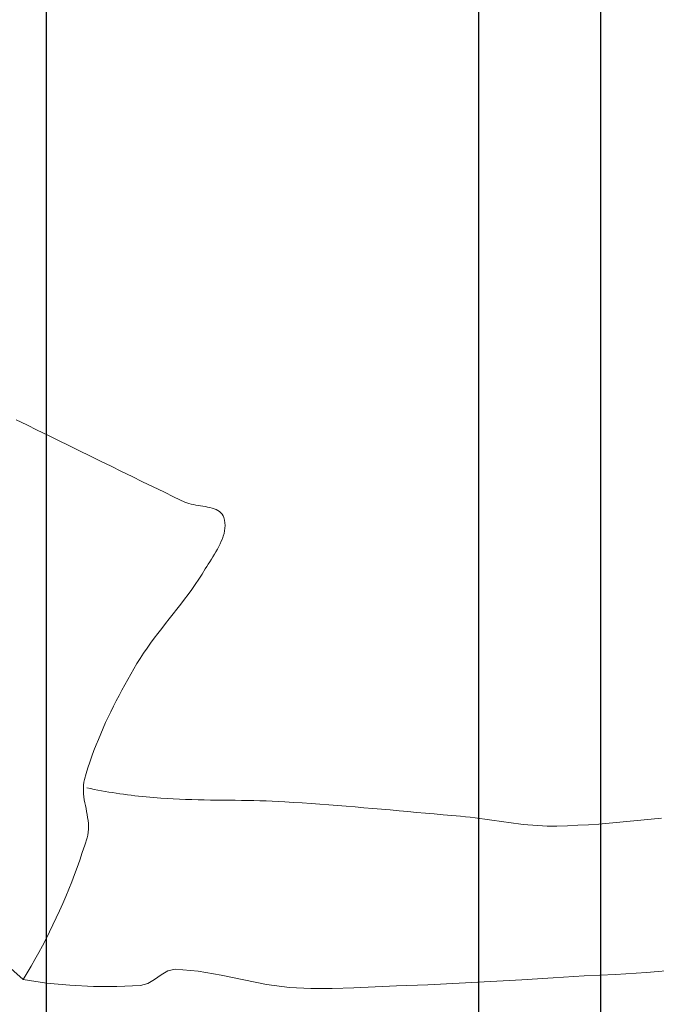
# Model space of a CAD drawing. Units: inches. Extents: x 2656 to 9931, y 1941 to 3068.
# Tile 9 of 46: x 2792 to 2811, y 2502 to 2533. Entities that reach past the tile are written whole.
import ezdxf

# ---------------------------------------------------------------- set-up
doc = ezdxf.new("R2010")
doc.units = ezdxf.units.IN
doc.layers.add('A-ANNO-DIMS', color=2, linetype='Continuous', lineweight=18)
doc.layers.add('A-FURN', color=8, linetype='Continuous', lineweight=13)
doc.styles.get("Standard").update_dxf_attribs({"font": 'arial.ttf'})
doc.dimstyles.new('ISO-25', dxfattribs={"dimtxt": 6, "dimasz": 2.5, "dimexe": 1.25, "dimexo": 0.625, "dimtad": 1, "dimdec": 0, "dimlunit": 3, "dimtxsty": 'Standard', "dimcen": 2.5, "dimadec": 0, "dimazin": 0, "dimtfac": 1, "dimtdec": 0, "dimtmove": 0, "dimatfit": 3, "dimfxl": 1, "dimarcsym": 0})

# ---------------------------------------------------------------- blocks, each defined once
blk = doc.blocks.new('BED-DOUBLE')
for p, q in [((38.504, 17.505), (38.175, 17.662)), ((38.832, 17.346), (38.504, 17.505)), ((39.16, 17.186), (38.832, 17.346)), ((39.488, 17.026), (39.16, 17.186)), ((39.816, 16.865), (39.488, 17.026)), ((40.143, 16.704), (39.816, 16.865)), ((40.47, 16.542), (40.143, 16.704)), ((40.797, 16.381), (40.47, 16.542)), ((41.125, 16.22), (40.797, 16.381)), ((41.452, 16.059), (41.125, 16.22)), ((41.78, 15.898), (41.452, 16.059)), ((42.107, 15.738), (41.78, 15.898)), ((42.436, 15.579), (42.107, 15.738)), ((42.764, 15.421), (42.436, 15.579)), ((43.094, 15.263), (42.764, 15.421)), ((43.424, 15.108), (43.094, 15.263)), ((43.485, 15.082), (43.424, 15.108)), ((43.55, 15.06), (43.485, 15.082)), ((43.618, 15.042), (43.55, 15.06)), ((43.689, 15.026), (43.618, 15.042)), ((43.762, 15.012), (43.689, 15.026)), ((43.836, 15), (43.762, 15.012)), ((43.91, 14.988), (43.836, 15)), ((43.985, 14.977), (43.91, 14.988)), ((44.059, 14.965), (43.985, 14.977)), ((44.131, 14.952), (44.059, 14.965)), ((44.201, 14.937), (44.131, 14.952)), ((44.269, 14.92), (44.201, 14.937)), ((44.333, 14.899), (44.269, 14.92)), ((44.394, 14.876), (44.333, 14.899)), ((44.45, 14.848), (44.394, 14.876)), ((44.501, 14.815), (44.45, 14.848)), ((44.545, 14.776), (44.501, 14.815)), ((44.584, 14.732), (44.545, 14.776)), ((44.615, 14.68), (44.584, 14.732)), ((44.638, 14.622), (44.615, 14.68)), ((44.658, 14.541), (44.638, 14.622)), ((44.67, 14.459), (44.658, 14.541)), ((44.673, 14.377), (44.67, 14.459)), ((44.617, 14.049), (44.64, 14.131)), ((44.64, 14.131), (44.658, 14.213)), ((44.658, 14.213), (44.669, 14.295)), ((44.669, 14.295), (44.673, 14.377)), ((44.478, 13.723), (44.519, 13.804)), ((44.519, 13.804), (44.556, 13.885)), ((44.556, 13.885), (44.588, 13.967)), ((44.588, 13.967), (44.617, 14.049)), ((44.294, 13.405), (44.342, 13.484)), ((44.342, 13.484), (44.389, 13.563)), ((44.389, 13.563), (44.435, 13.643)), ((44.435, 13.643), (44.478, 13.723)), ((44.103, 13.101), (44.149, 13.175)), ((44.149, 13.175), (44.197, 13.251)), ((44.197, 13.251), (44.246, 13.328)), ((44.246, 13.328), (44.294, 13.405)), ((43.958, 12.864), (44.058, 13.027)), ((44.058, 13.027), (44.103, 13.101)), ((43.747, 12.546), (43.854, 12.704)), ((43.854, 12.704), (43.958, 12.864)), ((43.524, 12.235), (43.637, 12.389)), ((43.637, 12.389), (43.747, 12.546)), ((43.293, 11.929), (43.409, 12.081)), ((43.409, 12.081), (43.524, 12.235)), ((43.057, 11.626), (43.175, 11.777)), ((43.175, 11.777), (43.293, 11.929)), ((42.82, 11.325), (42.938, 11.476)), ((42.938, 11.476), (43.057, 11.626)), ((42.585, 11.021), (42.702, 11.173)), ((42.702, 11.173), (42.82, 11.325)), ((42.356, 10.714), (42.469, 10.869)), ((42.469, 10.869), (42.585, 11.021)), ((42.136, 10.401), (42.245, 10.559)), ((42.245, 10.559), (42.356, 10.714)), ((41.93, 10.08), (42.031, 10.242)), ((42.031, 10.242), (42.136, 10.401)), ((41.739, 9.752), (41.832, 9.915)), ((41.832, 9.915), (41.93, 10.08)), ((41.555, 9.422), (41.647, 9.587)), ((41.647, 9.587), (41.739, 9.752)), ((41.377, 9.089), (41.465, 9.256)), ((41.465, 9.256), (41.555, 9.422)), ((41.204, 8.753), (41.289, 8.921)), ((41.289, 8.921), (41.377, 9.089)), ((41.038, 8.413), (41.12, 8.583)), ((41.12, 8.583), (41.204, 8.753)), ((40.958, 8.242), (41.038, 8.413)), ((40.805, 7.896), (40.88, 8.069)), ((40.88, 8.069), (40.958, 8.242)), ((40.661, 7.547), (40.732, 7.722)), ((40.732, 7.722), (40.805, 7.896)), ((40.529, 7.195), (40.594, 7.371)), ((40.594, 7.371), (40.661, 7.547)), ((40.467, 7.017), (40.529, 7.195)), ((40.353, 6.658), (40.408, 6.838)), ((40.408, 6.838), (40.467, 7.017)), ((40.281, 6.389), (40.301, 6.477)), ((40.301, 6.477), (40.353, 6.658)), ((40.264, 6.21), (40.269, 6.3)), ((40.264, 6.119), (40.264, 6.21)), ((40.269, 6.3), (40.281, 6.389)), ((40.368, 6.212), (40.482, 6.189)), ((40.482, 6.189), (40.596, 6.166)), ((40.596, 6.166), (40.711, 6.144)), ((40.711, 6.144), (40.826, 6.123)), ((40.27, 6.028), (40.264, 6.119)), ((40.281, 5.936), (40.27, 6.028)), ((40.294, 5.844), (40.281, 5.936)), ((40.31, 5.751), (40.294, 5.844)), ((40.826, 6.123), (40.941, 6.103)), ((40.941, 6.103), (41.056, 6.083)), ((41.056, 6.083), (41.171, 6.064)), ((41.171, 6.064), (41.286, 6.046)), ((41.286, 6.046), (41.402, 6.029)), ((41.402, 6.029), (41.517, 6.012)), ((41.517, 6.012), (41.633, 5.997)), ((41.633, 5.997), (41.749, 5.982)), ((41.749, 5.982), (41.864, 5.968)), ((41.864, 5.968), (41.98, 5.954)), ((41.98, 5.954), (42.096, 5.942)), ((42.096, 5.942), (42.213, 5.93)), ((42.213, 5.93), (42.329, 5.919)), ((42.329, 5.919), (42.445, 5.909)), ((42.445, 5.909), (42.561, 5.899)), ((42.561, 5.899), (42.677, 5.891)), ((42.677, 5.891), (42.87, 5.878)), ((42.87, 5.878), (43.062, 5.868)), ((43.062, 5.868), (43.254, 5.859)), ((43.254, 5.859), (43.447, 5.852)), ((43.447, 5.852), (43.639, 5.846)), ((43.639, 5.846), (43.832, 5.841)), ((43.832, 5.841), (44.024, 5.838)), ((44.024, 5.838), (44.217, 5.834)), ((44.217, 5.834), (44.41, 5.832)), ((44.41, 5.832), (44.602, 5.83)), ((44.602, 5.83), (44.795, 5.828)), ((44.795, 5.828), (44.988, 5.825)), ((44.988, 5.825), (45.18, 5.823)), ((45.18, 5.823), (45.373, 5.82)), ((40.328, 5.659), (40.31, 5.751)), ((40.347, 5.566), (40.328, 5.659)), ((40.365, 5.473), (40.347, 5.566)), ((45.373, 5.82), (45.566, 5.816)), ((45.566, 5.816), (45.758, 5.811)), ((45.758, 5.811), (45.951, 5.805)), ((45.951, 5.805), (46.143, 5.798)), ((46.143, 5.798), (46.336, 5.789)), ((46.336, 5.789), (46.528, 5.778)), ((46.528, 5.778), (46.802, 5.761)), ((46.802, 5.761), (47.076, 5.743)), ((47.076, 5.743), (47.35, 5.724)), ((47.35, 5.724), (47.624, 5.705)), ((47.624, 5.705), (47.898, 5.684)), ((47.898, 5.684), (48.172, 5.663)), ((48.172, 5.663), (48.445, 5.641)), ((48.445, 5.641), (48.719, 5.619)), ((48.719, 5.619), (48.993, 5.596)), ((48.993, 5.596), (49.266, 5.573)), ((49.266, 5.573), (49.54, 5.549)), ((49.54, 5.549), (49.813, 5.525)), ((49.813, 5.525), (50.087, 5.5)), ((40.382, 5.381), (40.365, 5.473)), ((40.398, 5.288), (40.382, 5.381)), ((40.411, 5.196), (40.398, 5.288)), ((50.087, 5.5), (50.36, 5.476)), ((50.36, 5.476), (50.634, 5.451)), ((50.634, 5.451), (50.907, 5.426)), ((50.907, 5.426), (51.181, 5.402)), ((51.181, 5.402), (51.454, 5.377)), ((51.454, 5.377), (51.728, 5.352)), ((51.728, 5.352), (52.002, 5.328)), ((52.002, 5.328), (52.151, 5.313)), ((52.151, 5.313), (52.301, 5.297)), ((52.301, 5.297), (52.451, 5.279)), ((52.451, 5.279), (52.601, 5.26)), ((52.601, 5.26), (52.75, 5.239)), ((52.75, 5.239), (52.9, 5.218)), ((52.9, 5.218), (53.05, 5.197)), ((57.605, 5.207), (57.93, 5.241)), ((57.93, 5.241), (58.256, 5.275)), ((40.42, 5.105), (40.411, 5.196)), ((40.416, 4.834), (40.424, 4.924)), ((40.424, 5.014), (40.42, 5.105)), ((40.424, 4.924), (40.424, 5.014)), ((53.05, 5.197), (53.199, 5.176)), ((53.199, 5.176), (53.349, 5.155)), ((53.349, 5.155), (53.498, 5.134)), ((53.498, 5.134), (53.648, 5.114)), ((53.648, 5.114), (53.798, 5.095)), ((53.798, 5.095), (53.947, 5.078)), ((53.947, 5.078), (54.097, 5.062)), ((54.097, 5.062), (54.247, 5.049)), ((54.247, 5.049), (54.397, 5.038)), ((54.397, 5.038), (54.547, 5.029)), ((54.547, 5.029), (54.697, 5.024)), ((54.697, 5.024), (54.847, 5.021)), ((54.847, 5.021), (54.998, 5.023)), ((54.998, 5.023), (55.324, 5.032)), ((55.324, 5.032), (55.651, 5.047)), ((55.651, 5.047), (55.977, 5.065)), ((55.977, 5.065), (56.303, 5.088)), ((56.303, 5.088), (56.628, 5.114)), ((56.628, 5.114), (56.954, 5.143)), ((56.954, 5.143), (57.279, 5.174)), ((57.279, 5.174), (57.605, 5.207)), ((40.307, 4.427), (40.38, 4.658)), ((40.38, 4.658), (40.402, 4.746)), ((40.402, 4.746), (40.416, 4.834)), ((40.232, 4.197), (40.307, 4.427)), ((40.154, 3.968), (40.232, 4.197)), ((39.988, 3.512), (40.072, 3.739)), ((40.072, 3.739), (40.154, 3.968)), ((39.901, 3.285), (39.988, 3.512)), ((39.811, 3.06), (39.901, 3.285)), ((39.623, 2.612), (39.718, 2.835)), ((39.718, 2.835), (39.811, 3.06)), ((39.524, 2.39), (39.623, 2.612)), ((39.319, 1.949), (39.423, 2.169)), ((39.423, 2.169), (39.524, 2.39)), ((39.213, 1.731), (39.319, 1.949)), ((39.103, 1.515), (39.213, 1.731)), ((38.876, 1.085), (38.991, 1.299)), ((38.991, 1.299), (39.103, 1.515)), ((37.459, 1.078), (38.392, 0.247)), ((38.759, 0.873), (38.876, 1.085)), ((38.517, 0.454), (38.639, 0.663)), ((38.639, 0.663), (38.759, 0.873)), ((38.392, 0.247), (38.517, 0.454)), ((42.478, 0.252), (42.684, 0.399)), ((42.684, 0.399), (42.897, 0.52)), ((42.897, 0.52), (43.125, 0.568)), ((43.125, 0.568), (43.84, 0.512)), ((43.84, 0.512), (44.549, 0.388)), ((44.549, 0.388), (45.256, 0.236)), ((54.881, 0.304), (55.85, 0.359)), ((55.85, 0.359), (56.819, 0.409)), ((56.819, 0.409), (57.788, 0.467)), ((57.788, 0.467), (58.754, 0.547)), ((38.392, 0.247), (39.115, 0.14)), ((39.115, 0.14), (39.844, 0.068)), ((39.844, 0.068), (40.575, 0.031)), ((40.575, 0.031), (41.307, 0.028)), ((41.307, 0.028), (42.038, 0.06)), ((42.038, 0.06), (42.266, 0.124)), ((42.266, 0.124), (42.478, 0.252)), ((45.256, 0.236), (45.964, 0.094)), ((45.964, 0.094), (46.677, 0.002)), ((46.677, 0.002), (47.342, -0.03)), ((48.675, -0.01), (49.342, 0.02)), ((49.342, 0.02), (50.009, 0.048)), ((50.009, 0.048), (50.984, 0.088)), ((50.984, 0.088), (51.958, 0.135)), ((51.958, 0.135), (52.933, 0.187)), ((52.933, 0.187), (53.907, 0.244)), ((53.907, 0.244), (54.881, 0.304)), ((47.342, -0.03), (48.009, -0.03)), ((48.009, -0.03), (48.675, -0.01))]:
    blk.add_line(p, q)
blk = doc.blocks.new('*D31')
at = {"layer": 'A-ANNO-DIMS', "color": 0, "lineweight": -2, "transparency": 16777216}
for p, q in [((2753.358, 2502.145), (2753.358, 2488.227)), ((2841.982, 2502.145), (2841.982, 2488.227)), ((2755.858, 2489.477), (2839.482, 2489.477)), ((2841.982, 2489.477), (2952.348, 2489.477))]:
    blk.add_line(p, q, dxfattribs=at)
at = {"layer": 'A-ANNO-DIMS', "color": 0, "transparency": 16777216}
for points in [[(2755.858, 2489.893), (2755.858, 2489.06), (2753.358, 2489.477)], [(2839.482, 2489.893), (2839.482, 2489.06), (2841.982, 2489.477)]]:
    blk.add_solid(points, dxfattribs=at)
at = {"layer": 'Defpoints', "color": 0, "transparency": 16777216}
for p in [(2753.358, 2502.77), (2841.982, 2502.77), (2841.982, 2489.477)]:
    blk.add_point(p, dxfattribs=at)
at = {"layer": 'A-ANNO-DIMS', "color": 0, "transparency": 16777216, "insert": (2898.415, 2493.206), "char_height": 6, "attachment_point": 5}
blk.add_mtext('DOUBLE BED 7\'-4 1/2" TYP.', dxfattribs=at)
blk = doc.blocks.new('*D113')
at = {"layer": 'A-ANNO-DIMS', "color": 0, "lineweight": -2, "transparency": 16777216}
for p, q in [((2752.157, 2300.725), (2752.157, 2674.45)), ((2809.769, 2300.725), (2809.769, 2674.45)), ((2754.657, 2673.2), (2807.269, 2673.2))]:
    blk.add_line(p, q, dxfattribs=at)
at = {"layer": 'A-ANNO-DIMS', "color": 0, "transparency": 16777216}
for points in [[(2754.657, 2673.617), (2754.657, 2672.784), (2752.157, 2673.2)], [(2807.269, 2673.617), (2807.269, 2672.784), (2809.769, 2673.2)]]:
    blk.add_solid(points, dxfattribs=at)
at = {"layer": 'Defpoints', "color": 0, "transparency": 16777216}
for p in [(2809.769, 2673.2), (2752.157, 2300.1), (2809.769, 2300.1)]:
    blk.add_point(p, dxfattribs=at)
at = {"layer": 'A-ANNO-DIMS', "color": 0, "transparency": 16777216, "insert": (2780.963, 2676.928), "char_height": 6, "attachment_point": 5}
blk.add_mtext('4\'-9 1/2"', dxfattribs=at)
blk = doc.blocks.new('*D114')
at = {"layer": 'A-ANNO-DIMS', "color": 0, "lineweight": -2, "transparency": 16777216}
for p, q in [((2809.769, 2300.725), (2809.769, 2674.45)), ((2851.877, 2300.725), (2851.877, 2674.45)), ((2812.269, 2673.2), (2849.377, 2673.2))]:
    blk.add_line(p, q, dxfattribs=at)
at = {"layer": 'A-ANNO-DIMS', "color": 0, "transparency": 16777216}
for points in [[(2812.269, 2673.617), (2812.269, 2672.784), (2809.769, 2673.2)], [(2849.377, 2673.617), (2849.377, 2672.784), (2851.877, 2673.2)]]:
    blk.add_solid(points, dxfattribs=at)
at = {"layer": 'Defpoints', "color": 0, "transparency": 16777216}
for p in [(2851.877, 2673.2), (2809.769, 2300.1), (2851.877, 2300.1)]:
    blk.add_point(p, dxfattribs=at)
at = {"layer": 'A-ANNO-DIMS', "color": 0, "transparency": 16777216, "insert": (2830.823, 2676.891), "char_height": 6, "attachment_point": 5}
blk.add_mtext('3\'-6"', dxfattribs=at)
blk = doc.blocks.new('*D129')
at = {"layer": 'A-ANNO-DIMS', "color": 0, "lineweight": -2, "transparency": 16777216}
for p, q in [((2752.157, 2601.146), (2752.157, 2009.273)), ((2777.587, 2557.74), (2777.587, 2009.273)), ((2754.657, 2010.523), (2775.087, 2010.523)), ((2777.587, 2010.523), (2811.37, 2010.523))]:
    blk.add_line(p, q, dxfattribs=at)
at = {"layer": 'A-ANNO-DIMS', "color": 0, "transparency": 16777216}
for points in [[(2754.657, 2010.939), (2754.657, 2010.106), (2752.157, 2010.523)], [(2775.087, 2010.939), (2775.087, 2010.106), (2777.587, 2010.523)]]:
    blk.add_solid(points, dxfattribs=at)
at = {"layer": 'Defpoints', "color": 0, "transparency": 16777216}
for p in [(2752.157, 2601.771), (2777.587, 2558.365), (2777.587, 2010.523)]:
    blk.add_point(p, dxfattribs=at)
at = {"layer": 'A-ANNO-DIMS', "color": 0, "transparency": 16777216, "insert": (2795.728, 2014.25), "char_height": 6, "attachment_point": 5}
blk.add_mtext('2\'-1 1/2"', dxfattribs=at)
blk = doc.blocks.new('*D132')
at = {"layer": 'A-ANNO-DIMS', "color": 0, "lineweight": -2, "transparency": 16777216}
for p, q in [((2763.467, 2366.557), (2763.467, 2674.45)), ((2805.965, 2366.557), (2805.965, 2674.45)), ((2765.967, 2673.2), (2803.465, 2673.2))]:
    blk.add_line(p, q, dxfattribs=at)
at = {"layer": 'A-ANNO-DIMS', "color": 0, "transparency": 16777216}
for points in [[(2765.967, 2673.617), (2765.967, 2672.784), (2763.467, 2673.2)], [(2803.465, 2673.617), (2803.465, 2672.784), (2805.965, 2673.2)]]:
    blk.add_solid(points, dxfattribs=at)
at = {"layer": 'Defpoints', "color": 0, "transparency": 16777216}
for p in [(2805.965, 2673.2), (2763.467, 2365.932), (2805.965, 2365.932)]:
    blk.add_point(p, dxfattribs=at)
at = {"layer": 'A-ANNO-DIMS', "color": 0, "transparency": 16777216, "insert": (2784.716, 2676.93), "char_height": 6, "attachment_point": 5}
blk.add_mtext('3\'-6 1/2"', dxfattribs=at)
blk = doc.blocks.new('*D134')
at = {"layer": 'A-ANNO-DIMS', "color": 0, "lineweight": -2, "transparency": 16777216}
for p, q in [((2752.157, 2300.725), (2752.157, 2674.45)), ((2763.467, 2347.433), (2763.467, 2674.45)), ((2754.657, 2673.2), (2760.967, 2673.2)), ((2763.467, 2673.2), (2801.809, 2673.2))]:
    blk.add_line(p, q, dxfattribs=at)
at = {"layer": 'A-ANNO-DIMS', "color": 0, "transparency": 16777216}
for points in [[(2754.657, 2673.617), (2754.657, 2672.784), (2752.157, 2673.2)], [(2760.967, 2673.617), (2760.967, 2672.784), (2763.467, 2673.2)]]:
    blk.add_solid(points, dxfattribs=at)
at = {"layer": 'Defpoints', "color": 0, "transparency": 16777216}
for p in [(2763.467, 2673.2), (2763.467, 2346.808), (2752.157, 2300.1)]:
    blk.add_point(p, dxfattribs=at)
at = {"layer": 'A-ANNO-DIMS', "color": 0, "transparency": 16777216, "insert": (2783.888, 2676.928), "char_height": 6, "attachment_point": 5}
blk.add_mtext('0\'-11 1/2"', dxfattribs=at)
blk = doc.blocks.new('*D136')
at = {"layer": 'A-ANNO-DIMS', "color": 0, "lineweight": -2, "transparency": 16777216}
for p, q in [((2765.357, 2375.042), (2765.357, 2674.45)), ((2779.142, 2375.042), (2779.142, 2674.45)), ((2767.857, 2673.2), (2776.642, 2673.2)), ((2779.142, 2673.2), (2798.277, 2673.2))]:
    blk.add_line(p, q, dxfattribs=at)
at = {"layer": 'A-ANNO-DIMS', "color": 0, "transparency": 16777216}
for points in [[(2767.857, 2673.617), (2767.857, 2672.784), (2765.357, 2673.2)], [(2776.642, 2673.617), (2776.642, 2672.784), (2779.142, 2673.2)]]:
    blk.add_solid(points, dxfattribs=at)
at = {"layer": 'Defpoints', "color": 0, "transparency": 16777216}
for p in [(2779.142, 2673.2), (2765.357, 2374.417), (2779.142, 2374.417)]:
    blk.add_point(p, dxfattribs=at)
at = {"layer": 'A-ANNO-DIMS', "color": 0, "transparency": 16777216, "insert": (2789.959, 2676.838), "char_height": 6, "attachment_point": 5}
blk.add_mtext('1\'-2"', dxfattribs=at)
blk = doc.blocks.new('*D137')
at = {"layer": 'A-ANNO-DIMS', "color": 0, "lineweight": -2, "transparency": 16777216}
for p, q in [((2779.142, 2375.042), (2779.142, 2674.45)), ((2792.516, 2375.042), (2792.516, 2674.45)), ((2781.642, 2673.2), (2790.016, 2673.2)), ((2792.516, 2673.2), (2825.632, 2673.2))]:
    blk.add_line(p, q, dxfattribs=at)
at = {"layer": 'A-ANNO-DIMS', "color": 0, "transparency": 16777216}
for points in [[(2781.642, 2673.617), (2781.642, 2672.784), (2779.142, 2673.2)], [(2790.016, 2673.617), (2790.016, 2672.784), (2792.516, 2673.2)]]:
    blk.add_solid(points, dxfattribs=at)
at = {"layer": 'Defpoints', "color": 0, "transparency": 16777216}
for p in [(2792.516, 2673.2), (2779.142, 2374.417), (2792.516, 2374.417)]:
    blk.add_point(p, dxfattribs=at)
at = {"layer": 'A-ANNO-DIMS', "color": 0, "transparency": 16777216, "insert": (2810.324, 2676.928), "char_height": 6, "attachment_point": 5}
blk.add_mtext('1\'-1 1/2"', dxfattribs=at)

msp = doc.modelspace()

# ---------------------------------------------------------------- block references
at = {"layer": 'A-FURN'}
msp.add_blockref('BED-DOUBLE', (2753.4, 2502.8), dxfattribs=at)

# ---------------------------------------------------------------- dimensions: what is measured, and where the dimension line sits
at = {"layer": 'A-ANNO-DIMS'}
for base, p1, p2, picture, middle in [((2809.769, 2673.2), (2752.157, 2300.1), (2809.769, 2300.1), '*D113', (2780.963, 2676.928)), ((2763.467, 2673.2), (2752.157, 2300.1), (2763.467, 2346.808), '*D134', (2783.888, 2676.928)), ((2805.965, 2673.2), (2763.467, 2365.932), (2805.965, 2365.932), '*D132', (2784.716, 2676.93)), ((2792.516, 2673.2), (2779.142, 2374.417), (2792.516, 2374.417), '*D137', (2810.324, 2676.928)), ((2779.142, 2673.2), (2765.357, 2374.417), (2779.142, 2374.417), '*D136', (2789.959, 2676.838)), ((2851.877, 2673.2), (2809.769, 2300.1), (2851.877, 2300.1), '*D114', (2830.823, 2676.891)), ((2777.587, 2010.523), (2752.157, 2601.771), (2777.587, 2558.365), '*D129', (2795.728, 2014.25))]:
    dim = msp.add_linear_dim(base=base, p1=p1, p2=p2, dimstyle='ISO-25', override={"dimdec": 1, "dimlfac": 1, "dimrnd": 0, "dimzin": 1, "dimdsep": 46, "dimlunit": 4, "dimfrac": 2}, dxfattribs=at)
    dim.commit()
    dim.dimension.update_dxf_attribs({"geometry": picture, "text_midpoint": middle})
dim = msp.add_linear_dim(base=(2841.982, 2489.477), p1=(2753.358, 2502.77), p2=(2841.982, 2502.77), text='DOUBLE BED <> TYP.', dimstyle='ISO-25', override={"dimdec": 1, "dimlfac": 1, "dimrnd": 0, "dimzin": 1, "dimdsep": 46, "dimlunit": 4, "dimfrac": 2}, dxfattribs=at)
dim.commit()
dim.dimension.update_dxf_attribs({"geometry": '*D31', "text_midpoint": (2898.415, 2493.206)})

doc.saveas('drawing.dxf')
